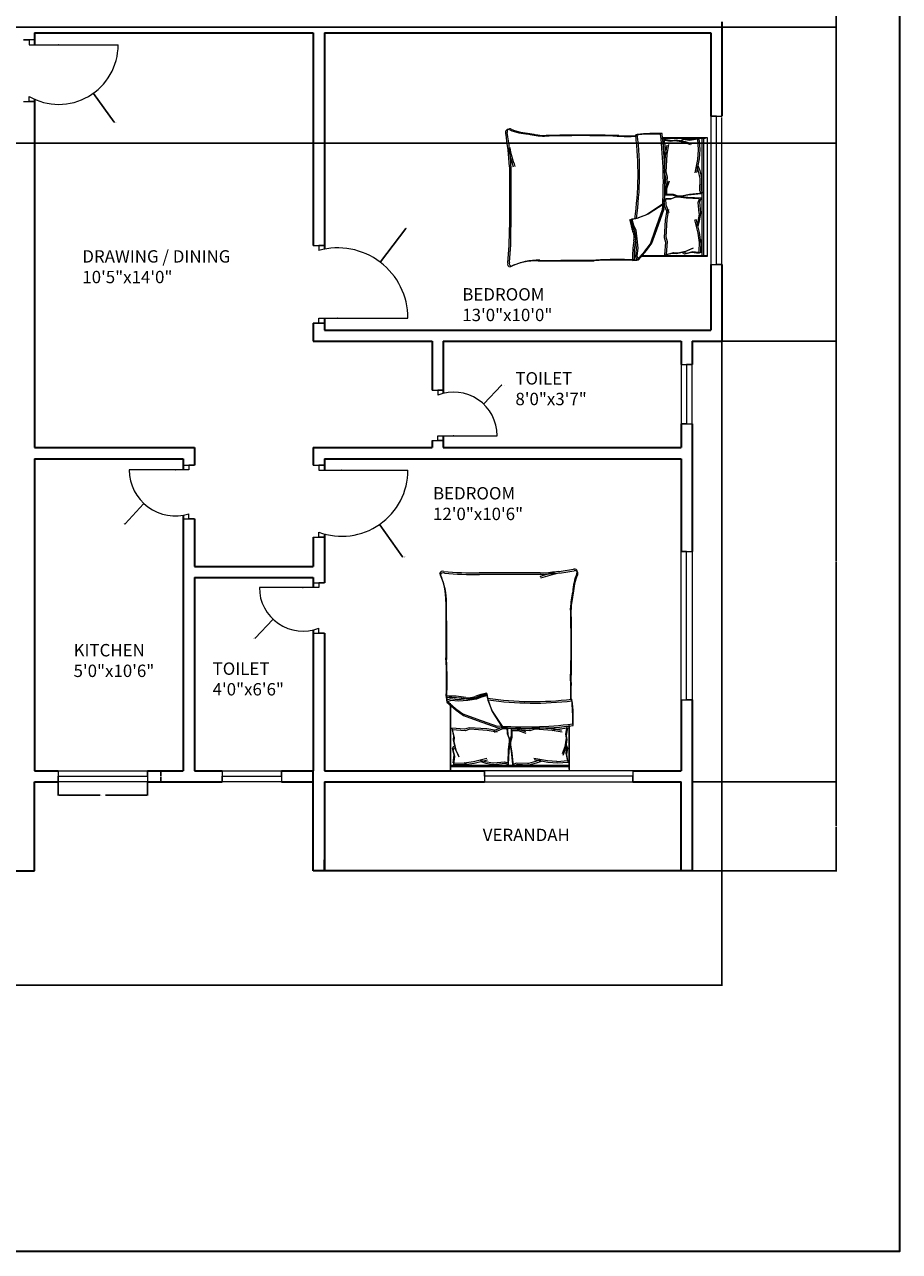
# Model space of a CAD drawing. Units: inches. Extents: x 1937 to 2996, y 1402 to 2323.
# Tile 9 of 10: x 2643 to 2996, y 1402 to 1897. Entities that reach past the tile are written whole.
import ezdxf

# ---------------------------------------------------------------- set-up
doc = ezdxf.new("R2010")
doc.units = ezdxf.units.IN
for name, color, linetype, lineweight in [('A-ANNO-DIMS', 2, 'Continuous', 18), ('A-ANNO-TTLB', 7, 'Continuous', 35), ('A-AREA-IDEN', 7, 'Continuous', 18), ('A-DOOR', 11, 'Continuous', 18), ('A-FURN', 8, 'Continuous', 13), ('A-GLAZ', 141, 'Continuous', 18), ('A-WALL', 7, 'Continuous', 35)]:
    doc.layers.add(name, color=color, linetype=linetype, lineweight=lineweight)
doc.styles.get("Standard").update_dxf_attribs({"font": 'arial.ttf'})
doc.dimstyles.get("Standard").update_dxf_attribs({"dimtxt": 0.18, "dimasz": 0.18, "dimexe": 0.18, "dimexo": 0.0625, "dimgap": 0.09, "dimtad": 0, "dimtih": 1, "dimtoh": 1, "dimdec": 4, "dimzin": 0, "dimdsep": 46, "dimtxsty": 'Standard', "dimcen": 0.09, "dimadec": 0, "dimazin": 0, "dimtfac": 1, "dimtdec": 4, "dimtofl": 0, "dimtmove": 0, "dimatfit": 3, "dimfxl": 1, "dimtolj": 1, "dimtzin": 0, "dimarcsym": 0})

# ---------------------------------------------------------------- blocks, each defined once
blk = doc.blocks.new('BED-DOUBLE')
for p, q in [((-24.01, -18.11), (-24.01, 0)), ((-24.01, -18.11), (-24.01, 0)), ((-24.01, 0), (24.01, 0)), ((23.78, 0), (23.78, -26.61)), ((23.78, 0), (23.78, -26.61)), ((24.01, 0), (24.01, -0.64)), ((-24.01, -1.53), (23.78, -1.53)), ((-24.01, -1.53), (23.78, -1.53)), ((-23.78, -18.75), (-23.78, -0.64)), ((-23.78, -18.75), (-23.78, -0.64)), ((-23.78, -2.17), (24.01, -2.17)), ((-23.78, -2.17), (24.01, -2.17)), ((-23.59, -3.34), (-19.3, -3.01)), ((-23.59, -3.34), (-19.31, -3.01)), ((-23.59, -3.32), (-23.01, -6.5)), ((-23.59, -3.32), (-23.01, -6.5)), ((-23.36, -3.98), (-19.08, -3.65)), ((-23.36, -3.98), (-19.08, -3.65)), ((-23.36, -3.96), (-22.78, -7.14)), ((-23.36, -3.96), (-22.78, -7.14)), ((-19.31, -3.01), (-19.2, -3.03)), ((-19.3, -3.01), (-19.2, -3.03)), ((-19.2, -3.03), (-15.38, -3.32)), ((-19.2, -3.03), (-15.38, -3.32)), ((-19.08, -3.65), (-18.97, -3.67)), ((-19.08, -3.65), (-18.97, -3.67)), ((-18.97, -3.67), (-15.15, -3.96)), ((-18.97, -3.67), (-15.15, -3.96)), ((-15.38, -3.32), (-9.88, -4.33)), ((-15.38, -3.32), (-9.88, -4.33)), ((-15.15, -3.96), (-9.65, -4.97)), ((-15.15, -3.96), (-9.65, -4.97)), ((-12.63, -3.75), (-10.61, -3.03)), ((-12.63, -3.75), (-10.61, -3.03)), ((-12.4, -4.39), (-10.38, -3.67)), ((-12.4, -4.39), (-10.38, -3.67)), ((-10.61, -3.03), (-7.71, -2.3)), ((-10.61, -3.03), (-7.71, -2.3)), ((-10.38, -3.67), (-7.49, -2.94)), ((-10.38, -3.67), (-7.49, -2.94)), ((-7.71, -2.3), (-7.39, -2.3)), ((-7.71, -2.3), (-7.39, -2.3)), ((-7.49, -2.94), (-7.16, -2.94)), ((-7.49, -2.94), (-7.16, -2.94)), ((-7.39, -2.3), (-2.95, -2.45)), ((-7.39, -2.3), (-2.95, -2.45)), ((-7.16, -2.94), (-2.72, -3.09)), ((-7.16, -2.94), (-2.72, -3.09)), ((-2.95, -2.45), (-1.5, -1.87)), ((-2.95, -2.45), (-1.5, -1.87)), ((-2.72, -3.09), (-1.27, -2.51)), ((-2.72, -3.09), (-1.27, -2.51)), ((-1.5, -1.87), (-0.92, -7.22)), ((-1.5, -1.87), (-0.92, -7.22)), ((-1.27, -2.51), (-0.7, -7.86)), ((-1.27, -2.51), (-0.7, -7.86)), ((0.49, -2.49), (0.25, -7.87)), ((0.49, -2.49), (0.25, -7.87)), ((0.72, -3.13), (0.48, -8.51)), ((0.72, -3.13), (0.48, -8.51)), ((1.97, -2.98), (0.49, -2.49)), ((1.97, -2.98), (0.49, -2.49)), ((2.2, -3.62), (0.72, -3.13)), ((2.2, -3.62), (0.72, -3.13)), ((6.4, -2.56), (1.97, -2.98)), ((6.4, -2.56), (1.97, -2.98)), ((6.63, -3.2), (2.2, -3.62)), ((6.63, -3.2), (2.2, -3.62)), ((6.72, -2.54), (6.4, -2.56)), ((6.72, -2.54), (6.4, -2.56)), ((6.95, -3.18), (6.63, -3.2)), ((6.95, -3.18), (6.63, -3.2)), ((9.65, -3.08), (6.72, -2.54)), ((9.65, -3.08), (6.72, -2.54)), ((9.88, -3.72), (6.95, -3.18)), ((9.88, -3.72), (6.95, -3.18)), ((14.43, -3.07), (9.01, -4.42)), ((14.43, -3.07), (9.01, -4.42)), ((14.66, -3.71), (9.24, -5.06)), ((14.66, -3.71), (9.24, -5.06)), ((11.72, -3.67), (9.65, -3.08)), ((11.72, -3.67), (9.65, -3.08)), ((11.94, -4.31), (9.88, -3.72)), ((11.94, -4.31), (9.88, -3.72)), ((18.23, -2.54), (14.43, -3.07)), ((18.23, -2.54), (14.43, -3.07)), ((18.46, -3.18), (14.66, -3.71)), ((18.46, -3.18), (14.66, -3.71)), ((22.63, -2.56), (17.23, -2.46)), ((17.23, -2.46), (18.23, -2.54)), ((22.63, -2.56), (17.23, -2.46)), ((17.23, -2.46), (18.23, -2.54)), ((22.86, -3.2), (17.45, -3.1)), ((17.45, -3.1), (18.46, -3.18)), ((22.86, -3.2), (17.45, -3.1)), ((17.45, -3.1), (18.46, -3.18)), ((22.63, -2.56), (22.25, -5.77)), ((22.63, -2.56), (22.25, -5.77)), ((22.86, -3.2), (22.48, -6.41)), ((22.86, -3.2), (22.48, -6.41)), ((24.01, -0.64), (24.01, -27.25)), ((24.01, -0.64), (24.01, -27.25)), ((-23.01, -6.5), (-23.45, -9.1)), ((-23.01, -6.5), (-23.45, -9.1)), ((-23.45, -9.1), (-22.87, -10.11)), ((-23.45, -9.1), (-22.87, -10.11)), ((-22.78, -7.14), (-23.22, -9.74)), ((-22.78, -7.14), (-23.22, -9.74)), ((-23.22, -9.74), (-22.64, -10.75)), ((-23.22, -9.74), (-22.64, -10.75)), ((-23.01, -12.57), (-22.43, -8.96)), ((-23.01, -12.57), (-22.43, -8.96)), ((-22.78, -13.21), (-22.2, -9.59)), ((-22.78, -13.21), (-22.21, -9.59)), ((-22.43, -8.96), (-21.42, -6.21)), ((-22.43, -8.96), (-21.42, -6.21)), ((-22.21, -9.59), (-21.19, -6.85)), ((-22.2, -9.59), (-21.19, -6.85)), ((-0.92, -7.22), (-0.35, -10.4)), ((-0.92, -7.22), (-0.35, -10.4)), ((-0.7, -7.86), (-0.12, -11.04)), ((-0.7, -7.86), (-0.12, -11.04)), ((0.25, -7.87), (-0.13, -11.08)), ((0.25, -7.87), (-0.13, -11.08)), ((0.48, -8.51), (0.1, -11.72)), ((0.48, -8.51), (0.1, -11.72)), ((21.83, -8.26), (20.64, -5.58)), ((21.82, -8.26), (20.64, -5.58)), ((22.05, -8.9), (20.87, -6.22)), ((22.05, -8.9), (20.87, -6.22)), ((22.63, -11.83), (21.82, -8.26)), ((22.63, -11.83), (21.83, -8.26)), ((22.86, -12.47), (22.05, -8.9)), ((22.86, -12.47), (22.05, -8.9)), ((22.25, -5.77), (22.84, -8.34)), ((22.25, -5.77), (22.84, -8.34)), ((22.84, -8.34), (22.33, -9.38)), ((22.84, -8.34), (22.33, -9.38)), ((22.48, -6.41), (23.07, -8.98)), ((22.48, -6.41), (23.07, -8.98)), ((23.07, -8.98), (22.56, -10.02)), ((23.07, -8.98), (22.56, -10.02)), ((-23.3, -17.34), (-22.72, -14.16)), ((-23.3, -17.34), (-22.72, -14.16)), ((-23.07, -17.98), (-22.49, -14.8)), ((-23.07, -17.98), (-22.49, -14.8)), ((-22.72, -14.16), (-23.01, -12.57)), ((-22.72, -14.16), (-23.01, -12.57)), ((-22.49, -14.8), (-22.78, -13.21)), ((-22.49, -14.8), (-22.78, -13.21)), ((-0.35, -11.7), (-0.92, -13.58)), ((-0.35, -11.7), (-0.92, -13.58)), ((-0.92, -13.58), (-0.92, -16.26)), ((-0.92, -13.58), (-0.92, -16.26)), ((-0.12, -12.34), (-0.7, -14.22)), ((-0.12, -12.34), (-0.7, -14.22)), ((-0.7, -14.22), (-0.7, -16.9)), ((-0.7, -14.22), (-0.7, -16.9)), ((-0.35, -10.4), (-0.35, -11.7)), ((-0.35, -10.4), (-0.35, -11.7)), ((-0.13, -11.08), (-0.05, -12.38)), ((-0.13, -11.08), (-0.05, -12.38)), ((-0.12, -11.04), (-0.12, -12.34)), ((-0.12, -11.04), (-0.12, -12.34)), ((-0.05, -12.38), (0.65, -14.22)), ((-0.05, -12.38), (0.65, -14.22)), ((0.1, -11.72), (0.18, -13.02)), ((0.1, -11.72), (0.18, -13.02)), ((0.18, -13.02), (0.87, -14.86)), ((0.18, -13.02), (0.87, -14.86)), ((0.65, -14.22), (0.81, -16.89)), ((0.65, -14.22), (0.81, -16.89)), ((0.87, -14.86), (1.04, -17.53)), ((0.87, -14.86), (1.04, -17.53)), ((22.44, -13.43), (22.63, -11.83)), ((22.44, -13.43), (22.63, -11.83)), ((23.21, -16.57), (22.44, -13.43)), ((23.21, -16.57), (22.44, -13.43)), ((22.67, -14.07), (22.86, -12.47)), ((22.67, -14.07), (22.86, -12.47)), ((23.44, -17.21), (22.67, -14.07)), ((23.44, -17.21), (22.67, -14.07)), ((-18.2, -16.62), (-23.3, -17.34)), ((-18.2, -16.62), (-23.3, -17.34)), ((-17.98, -17.26), (-23.07, -17.98)), ((-17.98, -17.26), (-23.07, -17.98)), ((-21.1, -15.63), (-17.07, -16.3)), ((-21.1, -15.63), (-17.07, -16.3)), ((-20.87, -16.27), (-16.84, -16.93)), ((-20.87, -16.27), (-16.84, -16.93)), ((-17.07, -16.3), (-18.2, -16.62)), ((-17.07, -16.3), (-18.2, -16.62)), ((-16.84, -16.93), (-17.98, -17.26)), ((-16.84, -16.93), (-17.98, -17.26)), ((-17.07, -16.3), (-10.06, -16.73)), ((-17.07, -16.3), (-10.06, -16.73)), ((-16.84, -16.93), (-9.83, -17.37)), ((-16.84, -16.93), (-9.83, -17.37)), ((-10.06, -16.73), (-8.1, -16.17)), ((-10.06, -16.73), (-8.1, -16.17)), ((-9.83, -17.37), (-7.87, -16.81)), ((-9.83, -17.37), (-7.87, -16.81)), ((-8.1, -16.17), (-2.97, -16.57)), ((-8.1, -16.17), (-2.97, -16.57)), ((-7.87, -16.81), (-2.74, -17.21)), ((-7.87, -16.81), (-2.74, -17.21)), ((-3.38, -16.26), (-6.53, -15.17)), ((-3.38, -16.26), (-6.53, -15.17)), ((-3.15, -16.9), (-6.3, -15.81)), ((-3.15, -16.9), (-6.3, -15.81)), ((-0.92, -16.26), (-3.38, -16.26)), ((-0.92, -16.26), (-3.38, -16.26)), ((-0.7, -16.9), (-3.15, -16.9)), ((-0.7, -16.9), (-3.15, -16.9)), ((0.81, -16.89), (3.27, -16.74)), ((0.81, -16.89), (3.27, -16.74)), ((1.04, -17.53), (3.49, -17.38)), ((1.04, -17.53), (3.49, -17.38)), ((2.77, -17.38), (6.97, -23.88)), ((2.77, -17.38), (6.96, -23.88)), ((3, -18.02), (7.19, -24.52)), ((3, -18.02), (7.19, -24.52)), ((3.27, -16.74), (6.34, -15.45)), ((3.27, -16.74), (6.34, -15.45)), ((3.49, -17.38), (6.56, -16.09)), ((3.49, -17.38), (6.56, -16.09)), ((13.16, -20.32), (4.82, -17.38)), ((13.16, -20.32), (4.82, -17.38)), ((13.39, -20.96), (5.05, -18.02)), ((13.39, -20.96), (5.05, -18.02)), ((5.08, -15.63), (9.11, -16.3)), ((5.08, -15.63), (9.11, -16.3)), ((5.31, -16.27), (9.34, -16.93)), ((5.31, -16.27), (9.34, -16.93)), ((9.11, -16.3), (16.12, -16.73)), ((9.11, -16.3), (16.12, -16.73)), ((9.34, -16.93), (16.35, -17.37)), ((9.34, -16.93), (16.35, -17.37)), ((16.12, -16.73), (18.08, -16.17)), ((16.12, -16.73), (18.08, -16.17)), ((16.35, -17.37), (18.31, -16.81)), ((16.35, -17.37), (18.31, -16.81)), ((18.08, -16.17), (23.21, -16.57)), ((18.08, -16.17), (23.21, -16.57)), ((18.31, -16.81), (23.44, -17.21)), ((18.31, -16.81), (23.44, -17.21)), ((6.96, -23.88), (8.67, -28.37)), ((6.97, -23.88), (8.67, -28.37)), ((7.19, -24.52), (8.9, -29)), ((7.19, -24.52), (8.9, -29)), ((18.74, -22.33), (13.16, -20.32)), ((18.74, -22.33), (13.16, -20.32)), ((18.96, -22.97), (13.39, -20.96)), ((18.96, -22.97), (13.39, -20.96)), ((21.68, -24.5), (18.74, -22.33)), ((21.68, -24.5), (18.74, -22.33)), ((21.91, -25.13), (18.96, -22.97)), ((21.91, -25.13), (18.96, -22.97)), ((25.38, -27.75), (21.68, -24.5)), ((25.38, -27.75), (21.68, -24.5)), ((8.67, -28.37), (8.98, -30.38)), ((8.67, -28.37), (8.98, -30.38)), ((8.9, -29), (9.21, -31.02)), ((8.9, -29), (9.21, -31.02)), ((11.46, -29.76), (13.47, -28.83)), ((11.46, -29.76), (13.47, -28.83)), ((11.68, -30.4), (13.7, -29.47)), ((11.68, -30.4), (13.7, -29.47)), ((13.47, -28.83), (16.88, -28.37)), ((13.47, -28.83), (16.88, -28.37)), ((13.7, -29.47), (17.11, -29)), ((13.7, -29.47), (17.1, -29)), ((16.88, -28.37), (20.75, -28.06)), ((16.88, -28.37), (20.75, -28.06)), ((17.1, -29), (20.98, -28.69)), ((17.11, -29), (20.98, -28.69)), ((20.75, -28.06), (23.85, -28.37)), ((20.75, -28.06), (23.85, -28.37)), ((20.98, -28.69), (24.07, -29)), ((20.98, -28.69), (24.07, -29)), ((25.61, -28.39), (21.91, -25.13)), ((25.61, -28.39), (21.91, -25.13)), ((23.85, -28.37), (25.38, -27.75)), ((23.85, -28.37), (25.38, -27.75)), ((24.07, -29), (25.61, -28.39)), ((24.07, -29), (25.61, -28.39)), ((25.46, -29.49), (25.38, -27.75, 3.87)), ((25.46, -29.49), (25.38, -27.75, 3.87)), ((25.69, -30.13), (25.61, -28.39, 3.87)), ((25.69, -30.13), (25.61, -28.39, 3.87)), ((8.98, -30.38), (11.46, -29.76)), ((8.98, -30.38), (11.46, -29.76)), ((9.21, -31.02), (11.68, -30.4)), ((9.21, -31.02), (11.68, -30.4)), ((-12.42, -79.25), (12.19, -79.25)), ((-12.42, -79.25), (12.19, -79.25)), ((-12.19, -79.88), (12.42, -79.88)), ((-12.19, -79.88), (12.42, -79.88))]:
    blk.add_line(p, q)
for centre, radius, start, end in [((57.68, -20.1), 83.31, 178.7218, 185.604), ((57.68, -20.1), 83.31, 178.7218, 185.604), ((-6.13, -182.05), 164.97, 86.0865, 96.7821), ((-6.13, -182.05), 164.97, 86.0865, 96.7821), ((57.91, -20.74), 83.31, 178.7218, 185.604), ((57.91, -20.74), 83.31, 178.7218, 185.604), ((-5.9, -182.69), 164.97, 86.0865, 96.7821), ((-5.9, -182.69), 164.97, 86.0865, 96.7821), ((-9.73, -156.32), 129.02, 81.7845, 96.9006), ((-9.73, -156.32), 129.02, 81.7845, 96.9006), ((-9.5, -156.96), 129.02, 81.7845, 96.9006), ((-9.5, -156.96), 129.02, 81.7845, 96.9006), ((-194.79, -31.17), 170.11, 358.4762, 1.0082), ((-194.79, -31.17), 170.11, 358.4762, 1.0082), ((-194.56, -31.81), 170.11, 358.4762, 1.0082), ((-194.56, -31.81), 170.11, 358.4762, 1.0082), ((3.67, -1.48), 29.65, 280.6617, 289.8806), ((3.67, -1.48), 29.65, 280.6617, 289.8806), ((16.26, -35.07), 6.22, 78.6608, 113.7384), ((16.26, -35.07), 6.22, 78.6608, 113.7384), ((16.49, -35.71), 6.22, 78.6608, 113.7384), ((16.49, -35.71), 6.22, 78.6608, 113.7384), ((23.84, 6.66), 36.18, 259.8763, 272.5657), ((23.84, 6.66), 36.18, 259.8763, 272.5657), ((24.07, 6.02), 36.18, 259.8763, 272.5657), ((24.07, 6.02), 36.18, 259.8763, 272.5657), ((154.78, -36.32), 129.5, 176.9791, 183.8365), ((154.78, -36.32), 129.5, 176.9791, 183.8365), ((9.15, -30.44), 0.185, 160.2464, 271.1377), ((9.15, -30.44), 0.185, 160.2464, 271.1377), ((9.38, -31.08), 0.185, 160.2464, 271.1377), ((9.38, -31.08), 0.185, 160.2464, 271.1377), ((3.9, -2.12), 29.65, 280.6617, 289.8806), ((3.9, -2.12), 29.65, 280.6617, 289.8806), ((155.01, -36.95), 129.5, 176.9791, 183.8365), ((155.01, -36.95), 129.5, 176.9791, 183.8365), ((457.34, -50.61), 482.31, 178.2277, 181.7185), ((457.34, -50.61), 482.31, 178.2277, 181.7185), ((457.57, -51.25), 482.31, 178.2277, 181.7185), ((457.57, -51.25), 482.31, 178.2277, 181.7185), ((-4536.23, -67.82), 4561.86, 0.00217, 0.28689), ((-4536.23, -67.82), 4561.86, 0.00217, 0.28689), ((-4536, -68.46), 4561.86, 0.00217, 0.28689), ((-4536, -68.46), 4561.86, 0.00217, 0.28689), ((-54.38, -64.52), 29.63, 346.0648, 358.9113), ((-54.38, -64.52), 29.63, 346.0648, 358.9113), ((-54.16, -65.15), 29.63, 346.0648, 358.9113), ((-54.16, -65.15), 29.63, 346.0648, 358.9113), ((48.67, -68.67), 23.07, 177.4714, 206.4681), ((48.67, -68.67), 23.07, 177.4714, 206.4681), ((48.9, -69.31), 23.07, 177.4714, 206.4681), ((48.9, -69.31), 23.07, 177.4714, 206.4681), ((-49.14, -70.28), 23.56, 337.9751, 356.652), ((-49.14, -70.28), 23.56, 337.9751, 356.652), ((-48.92, -70.91), 23.56, 337.9751, 356.652), ((-48.92, -70.91), 23.56, 337.9751, 356.652), ((-26.4, -79.72), 1.09, 146.1736, 293.4781), ((-26.4, -79.72), 1.09, 146.1736, 293.4781), ((-6.06, -200.84), 121.76, 92.9958, 99.4091), ((-6.06, -200.84), 121.76, 92.9958, 99.4091), ((-44.71, 23.71), 106.46, 283.3832, 287.7053), ((-44.71, 23.71), 106.46, 283.3832, 287.7053), ((-44.48, 23.07), 106.46, 283.3832, 287.7053), ((-44.48, 23.07), 106.46, 283.3832, 287.7053), ((13.67, -212.28), 133.04, 84.4998, 90.6351), ((13.67, -212.28), 133.04, 84.4998, 90.6351), ((26.93, -78.87), 1.1, 242.6588, 356.02), ((26.93, -78.87), 1.1, 242.6588, 356.02), ((-26.17, -80.36), 1.09, 146.1736, 293.4781), ((-26.17, -80.36), 1.09, 146.1736, 293.4781), ((-5.83, -201.48), 121.76, 92.9958, 99.4091), ((-5.83, -201.48), 121.76, 92.9958, 99.4091), ((13.9, -212.92), 133.04, 84.4998, 90.6351), ((13.9, -212.92), 133.04, 84.4998, 90.6351), ((27.15, -79.51), 1.1, 242.6588, 356.02), ((27.15, -79.51), 1.1, 242.6588, 356.02)]:
    blk.add_arc(centre, radius, start, end)
blk = doc.blocks.new('WINDOW-60IN')
for p, q in [((0, 2.25), (0, -2.25)), ((0, 2.25), (60, 2.25)), ((0, -2.25), (0, 0)), ((0, 0), (60, 0)), ((60, 0), (60, 2.25)), ((60, 2.25), (60, -2.25)), ((60, -2.25), (0, -2.25))]:
    blk.add_line(p, q)
blk = doc.blocks.new('WINDOW-24IN')
for p, q in [((0, -2.25), (0, 2.25)), ((0, 2.25), (0, 0)), ((24, 2.25), (0, 2.25)), ((0, 0), (24, 0)), ((24, -2.25), (24, 2.25)), ((24, 0), (24, -2.25)), ((0, -2.25), (24, -2.25))]:
    blk.add_line(p, q)
blk = doc.blocks.new('WINDOW-36IN')
for p, q in [((0, 2.25), (0, -2.25)), ((0, 2.25), (36, 2.25)), ((36, 0), (36, 2.25)), ((36, 2.25), (36, -2.25)), ((0, -2.25), (0, 0)), ((0, 0), (36, 0)), ((36, -2.25), (0, -2.25))]:
    blk.add_line(p, q)
blk = doc.blocks.new('*D15')
at = {"layer": 'A-ANNO-DIMS', "color": 0, "lineweight": -2, "transparency": 16777216}
for p, q in [((2656.2, 1591.24), (2656.2, 1585.73)), ((2692.2, 1591.24), (2692.2, 1585.73)), ((2656.38, 1585.91), (2673.09, 1585.91)), ((2692.02, 1585.91), (2675.32, 1585.91))]:
    blk.add_line(p, q, dxfattribs=at)
at = {"layer": 'A-ANNO-DIMS', "color": 0, "transparency": 16777216}
for points in [[(2656.38, 1585.94), (2656.38, 1585.88), (2656.2, 1585.91)], [(2692.02, 1585.94), (2692.02, 1585.88), (2692.2, 1585.91)]]:
    blk.add_solid(points, dxfattribs=at)
at = {"layer": 'Defpoints', "color": 0, "transparency": 16777216}
for p in [(2656.2, 1591.31), (2692.2, 1591.31), (2692.2, 1585.91)]:
    blk.add_point(p, dxfattribs=at)
at = {"layer": 'A-ANNO-DIMS', "color": 0, "transparency": 16777216, "insert": (2674.2, 1585.91), "char_height": 0.18, "attachment_point": 5}
blk.add_mtext('\\A1;WINDOW 36 TYP.', dxfattribs=at)
blk = doc.blocks.new('*D16')
at = {"layer": 'A-ANNO-DIMS', "color": 0, "lineweight": -2, "transparency": 16777216}
for p, q in [((2692.27, 1595.81), (2697.78, 1595.81)), ((2692.27, 1591.31), (2697.78, 1591.31)), ((2697.6, 1595.63), (2697.6, 1593.74)), ((2697.6, 1591.49), (2697.6, 1593.37))]:
    blk.add_line(p, q, dxfattribs=at)
at = {"layer": 'A-ANNO-DIMS', "color": 0, "transparency": 16777216}
for points in [[(2697.57, 1595.63), (2697.63, 1595.63), (2697.6, 1595.81)], [(2697.57, 1591.49), (2697.63, 1591.49), (2697.6, 1591.31)]]:
    blk.add_solid(points, dxfattribs=at)
at = {"layer": 'Defpoints', "color": 0, "transparency": 16777216}
for p in [(2692.2, 1595.81), (2697.6, 1595.81), (2692.2, 1591.31)]:
    blk.add_point(p, dxfattribs=at)
at = {"layer": 'A-ANNO-DIMS', "color": 0, "transparency": 16777216, "insert": (2697.6, 1593.56), "char_height": 0.18, "attachment_point": 5}
blk.add_mtext('\\A1;5 TYP.', dxfattribs=at)
blk = doc.blocks.new('*D23')
at = {"layer": 'A-ANNO-DIMS', "color": 0, "lineweight": -2, "transparency": 16777216}
for p, q in [((2010.65, 1769.24), (2010.65, 1508.98)), ((2924.15, 1769.24), (2924.15, 1508.98)), ((2010.83, 1509.16), (2467, 1509.16)), ((2923.97, 1509.16), (2467.79, 1509.16))]:
    blk.add_line(p, q, dxfattribs=at)
at = {"layer": 'A-ANNO-DIMS', "color": 0, "transparency": 16777216}
for points in [[(2010.83, 1509.19), (2010.83, 1509.13), (2010.65, 1509.16)], [(2923.97, 1509.19), (2923.97, 1509.13), (2924.15, 1509.16)]]:
    blk.add_solid(points, dxfattribs=at)
at = {"layer": 'Defpoints', "color": 0, "transparency": 16777216}
for p in [(2010.65, 1769.31), (2924.15, 1769.31), (2924.15, 1509.16)]:
    blk.add_point(p, dxfattribs=at)
at = {"layer": 'A-ANNO-DIMS', "color": 0, "transparency": 16777216, "insert": (2467.4, 1509.16), "char_height": 0.18, "attachment_point": 5}
blk.add_mtext('\\A1;913.5', dxfattribs=at)
blk = doc.blocks.new('*D37')
at = {"layer": 'A-ANNO-DIMS', "color": 0, "lineweight": -2, "transparency": 16777216}
for p, q in [((2455.84, 1896.06), (2970.48, 1896.06)), ((2970.3, 1895.88), (2970.3, 1872.86)), ((2970.3, 1849.49), (2970.3, 1872.5)), ((2455.84, 1849.31), (2970.48, 1849.31))]:
    blk.add_line(p, q, dxfattribs=at)
at = {"layer": 'A-ANNO-DIMS', "color": 0, "transparency": 16777216}
for points in [[(2970.27, 1895.88), (2970.33, 1895.88), (2970.3, 1896.06)], [(2970.27, 1849.49), (2970.33, 1849.49), (2970.3, 1849.31)]]:
    blk.add_solid(points, dxfattribs=at)
at = {"layer": 'Defpoints', "color": 0, "transparency": 16777216}
for p in [(2455.77, 1896.06), (2455.77, 1849.31), (2970.3, 1849.31)]:
    blk.add_point(p, dxfattribs=at)
at = {"layer": 'A-ANNO-DIMS', "color": 0, "transparency": 16777216, "insert": (2970.3, 1872.68), "char_height": 0.18, "attachment_point": 5}
blk.add_mtext('\\A1;46.75', dxfattribs=at)
blk = doc.blocks.new('*D39')
at = {"layer": 'A-ANNO-DIMS', "color": 0, "lineweight": -2, "transparency": 16777216}
for p, q in [((2912.21, 1591.31), (2970.48, 1591.31)), ((2970.3, 1591.13), (2970.3, 1573.49)), ((2970.3, 1555.49), (2970.3, 1573.12)), ((2912.21, 1555.31), (2970.48, 1555.31))]:
    blk.add_line(p, q, dxfattribs=at)
at = {"layer": 'A-ANNO-DIMS', "color": 0, "transparency": 16777216}
for points in [[(2970.27, 1591.13), (2970.33, 1591.13), (2970.3, 1591.31)], [(2970.27, 1555.49), (2970.33, 1555.49), (2970.3, 1555.31)]]:
    blk.add_solid(points, dxfattribs=at)
at = {"layer": 'Defpoints', "color": 0, "transparency": 16777216}
for p in [(2912.15, 1591.31), (2970.3, 1591.31), (2912.15, 1555.31)]:
    blk.add_point(p, dxfattribs=at)
at = {"layer": 'A-ANNO-DIMS', "color": 0, "transparency": 16777216, "insert": (2970.3, 1573.31), "char_height": 0.18, "attachment_point": 5}
blk.add_mtext('\\A1;36', dxfattribs=at)
blk = doc.blocks.new('*D40')
at = {"layer": 'A-ANNO-DIMS', "color": 0, "lineweight": -2, "transparency": 16777216}
for p, q in [((2912.21, 1769.31), (2970.48, 1769.31)), ((2970.3, 1769.13), (2970.3, 1680.49)), ((2970.3, 1591.49), (2970.3, 1680.12)), ((2912.21, 1591.31), (2970.48, 1591.31))]:
    blk.add_line(p, q, dxfattribs=at)
at = {"layer": 'A-ANNO-DIMS', "color": 0, "transparency": 16777216}
for points in [[(2970.27, 1769.13), (2970.33, 1769.13), (2970.3, 1769.31)], [(2970.27, 1591.49), (2970.33, 1591.49), (2970.3, 1591.31)]]:
    blk.add_solid(points, dxfattribs=at)
at = {"layer": 'Defpoints', "color": 0, "transparency": 16777216}
for p in [(2912.15, 1769.31), (2970.3, 1769.31), (2912.15, 1591.31)]:
    blk.add_point(p, dxfattribs=at)
at = {"layer": 'A-ANNO-DIMS', "color": 0, "transparency": 16777216, "insert": (2970.3, 1680.31), "char_height": 0.18, "attachment_point": 5}
blk.add_mtext('\\A1;178', dxfattribs=at)
blk = doc.blocks.new('*D41')
at = {"layer": 'A-ANNO-DIMS', "color": 0, "lineweight": -2, "transparency": 16777216}
for p, q in [((2924.21, 2022.81), (2970.48, 2022.81)), ((2970.3, 2022.63), (2970.3, 1896.24)), ((2970.3, 1769.49), (2970.3, 1895.87)), ((2924.21, 1769.31), (2970.48, 1769.31))]:
    blk.add_line(p, q, dxfattribs=at)
at = {"layer": 'A-ANNO-DIMS', "color": 0, "transparency": 16777216}
for points in [[(2970.27, 2022.63), (2970.33, 2022.63), (2970.3, 2022.81)], [(2970.27, 1769.49), (2970.33, 1769.49), (2970.3, 1769.31)]]:
    blk.add_solid(points, dxfattribs=at)
at = {"layer": 'Defpoints', "color": 0, "transparency": 16777216}
for p in [(2924.15, 2022.81), (2970.3, 2022.81), (2924.15, 1769.31)]:
    blk.add_point(p, dxfattribs=at)
at = {"layer": 'A-ANNO-DIMS', "color": 0, "transparency": 16777216, "insert": (2970.3, 1896.06), "char_height": 0.18, "attachment_point": 5}
blk.add_mtext('\\A1;253.5', dxfattribs=at)
blk = doc.blocks.new('*D65')
at = {"layer": 'A-ANNO-DIMS', "color": 0, "lineweight": -2, "transparency": 16777216}
for p, q in [((2796.48, 1814.77), (2786.29, 1801.35)), ((2796.66, 1814.77), (2796.48, 1814.77)), ((2768.92, 1778.61), (2769.1, 1778.61)), ((2769.01, 1778.52), (2769.01, 1778.7))]:
    blk.add_line(p, q, dxfattribs=at)
at = {"layer": 'A-ANNO-DIMS', "color": 0, "transparency": 16777216}
blk.add_solid([(2786.27, 1801.37), (2786.31, 1801.33), (2786.18, 1801.21)], dxfattribs=at)
at = {"layer": 'Defpoints', "color": 0, "transparency": 16777216}
for p in [(2786.18, 1801.21), (2769.01, 1778.61)]:
    blk.add_point(p, dxfattribs=at)
at = {"layer": 'A-ANNO-DIMS', "color": 0, "transparency": 16777216, "insert": (2797.21, 1814.77), "char_height": 0.18, "attachment_point": 5}
blk.add_mtext('\\A1;R28.385', dxfattribs=at)
blk = doc.blocks.new('*D69')
at = {"layer": 'A-ANNO-DIMS', "color": 0, "lineweight": -2, "transparency": 16777216}
for p, q in [((2770.56, 1717.24), (2770.74, 1717.24)), ((2770.65, 1717.15), (2770.65, 1717.33)), ((2795.12, 1682.13), (2786.05, 1695.15)), ((2795.3, 1682.13), (2795.12, 1682.13))]:
    blk.add_line(p, q, dxfattribs=at)
at = {"layer": 'A-ANNO-DIMS', "color": 0, "transparency": 16777216}
blk.add_solid([(2786.07, 1695.17), (2786.02, 1695.13), (2785.95, 1695.3)], dxfattribs=at)
at = {"layer": 'Defpoints', "color": 0, "transparency": 16777216}
for p in [(2770.65, 1717.24), (2785.95, 1695.3)]:
    blk.add_point(p, dxfattribs=at)
at = {"layer": 'A-ANNO-DIMS', "color": 0, "transparency": 16777216, "insert": (2795.85, 1682.13), "char_height": 0.18, "attachment_point": 5}
blk.add_mtext('\\A1;R26.747', dxfattribs=at)
blk = doc.blocks.new('*D87')
at = {"layer": 'A-ANNO-DIMS', "color": 0, "lineweight": -2, "transparency": 16777216}
for p, q in [((2703.38, 1717.27), (2703.56, 1717.27)), ((2703.47, 1717.18), (2703.47, 1717.36)), ((2683.18, 1695.56), (2690.66, 1703.57)), ((2683, 1695.56), (2683.18, 1695.56))]:
    blk.add_line(p, q, dxfattribs=at)
at = {"layer": 'A-ANNO-DIMS', "color": 0, "transparency": 16777216}
blk.add_solid([(2690.64, 1703.59), (2690.69, 1703.55), (2690.79, 1703.7)], dxfattribs=at)
at = {"layer": 'Defpoints', "color": 0, "transparency": 16777216}
for p in [(2703.47, 1717.27), (2690.79, 1703.7)]:
    blk.add_point(p, dxfattribs=at)
at = {"layer": 'A-ANNO-DIMS', "color": 0, "transparency": 16777216, "insert": (2682.52, 1695.56), "char_height": 0.18, "attachment_point": 5}
blk.add_mtext('\\A1;R18.57', dxfattribs=at)
blk = doc.blocks.new('*D88')
at = {"layer": 'A-ANNO-DIMS', "color": 0, "lineweight": -2, "transparency": 16777216}
for p, q in [((2754.87, 1669.75), (2755.05, 1669.75)), ((2754.96, 1669.66), (2754.96, 1669.84)), ((2735.69, 1649.3), (2742.79, 1656.84)), ((2735.51, 1649.3), (2735.69, 1649.3))]:
    blk.add_line(p, q, dxfattribs=at)
at = {"layer": 'A-ANNO-DIMS', "color": 0, "transparency": 16777216}
blk.add_solid([(2742.77, 1656.86), (2742.81, 1656.82), (2742.92, 1656.97)], dxfattribs=at)
at = {"layer": 'Defpoints', "color": 0, "transparency": 16777216}
for p in [(2754.96, 1669.75), (2742.92, 1656.97)]:
    blk.add_point(p, dxfattribs=at)
at = {"layer": 'A-ANNO-DIMS', "color": 0, "transparency": 16777216, "insert": (2735.03, 1649.3), "char_height": 0.18, "attachment_point": 5}
blk.add_mtext('\\A1;R17.56', dxfattribs=at)
blk = doc.blocks.new('*D89')
at = {"layer": 'A-ANNO-DIMS', "color": 0, "lineweight": -2, "transparency": 16777216}
for p, q in [((2835.17, 1751.56), (2828.03, 1744.03)), ((2835.35, 1751.56), (2835.17, 1751.56)), ((2815.7, 1731.12), (2815.88, 1731.12)), ((2815.79, 1731.03), (2815.79, 1731.21))]:
    blk.add_line(p, q, dxfattribs=at)
at = {"layer": 'A-ANNO-DIMS', "color": 0, "transparency": 16777216}
blk.add_solid([(2828.01, 1744.05), (2828.05, 1744.01), (2827.9, 1743.9)], dxfattribs=at)
at = {"layer": 'Defpoints', "color": 0, "transparency": 16777216}
for p in [(2827.9, 1743.9), (2815.79, 1731.12)]:
    blk.add_point(p, dxfattribs=at)
at = {"layer": 'A-ANNO-DIMS', "color": 0, "transparency": 16777216, "insert": (2835.9, 1751.56), "char_height": 0.18, "attachment_point": 5}
blk.add_mtext('\\A1;R17.604', dxfattribs=at)
blk = doc.blocks.new('*D90')
at = {"layer": 'A-ANNO-DIMS', "color": 0, "lineweight": -2, "transparency": 16777216}
for p, q in [((2656.29, 1888.95), (2656.47, 1888.95)), ((2656.38, 1888.86), (2656.38, 1889.04)), ((2678.8, 1857.75), (2670.5, 1869.3)), ((2678.98, 1857.75), (2678.8, 1857.75))]:
    blk.add_line(p, q, dxfattribs=at)
at = {"layer": 'A-ANNO-DIMS', "color": 0, "transparency": 16777216}
blk.add_solid([(2670.52, 1869.32), (2670.48, 1869.29), (2670.4, 1869.45)], dxfattribs=at)
at = {"layer": 'Defpoints', "color": 0, "transparency": 16777216}
for p in [(2656.38, 1888.95), (2670.4, 1869.45)]:
    blk.add_point(p, dxfattribs=at)
at = {"layer": 'A-ANNO-DIMS', "color": 0, "transparency": 16777216, "insert": (2679.53, 1857.75), "char_height": 0.18, "attachment_point": 5}
blk.add_mtext('\\A1;R24.017', dxfattribs=at)

msp = doc.modelspace()

# ---------------------------------------------------------------- linework, layer by layer
at = {"layer": 'A-ANNO-TTLB'}
msp.add_lwpolyline([(1937.1125, 2323.2883), (2995.8132, 2323.2883), (2995.8132, 1401.6335), (1937.1125, 1401.6335)], close=True, dxfattribs=at)
at = {"layer": 'A-DOOR'}
for p, q in [((2646.6473, 1890.9534), (2642.1473, 1890.9534)), ((2642.1473, 1890.9534), (2644.3973, 1890.9534)), ((2644.3973, 1890.9534), (2644.3973, 1888.9534)), ((2644.3973, 1888.9534), (2680.3973, 1888.9534)), ((2642.1473, 1866.1389), (2646.6473, 1866.1389)), ((2644.3973, 1866.1389), (2644.3973, 1868.1389)), ((2646.6473, 1866.1389), (2644.3973, 1866.1389)), ((2759.1473, 1807.9501), (2763.6473, 1807.9501)), ((2763.6473, 1807.9501), (2761.3973, 1807.9501)), ((2761.3973, 1807.9501), (2761.3973, 1805.9501)), ((2763.6473, 1776.6052), (2759.1473, 1776.6052)), ((2759.1473, 1776.6052), (2763.6473, 1776.6052)), ((2761.3973, 1776.6052), (2761.3973, 1778.6052)), ((2761.3973, 1778.6052), (2797.3973, 1778.6052)), ((2763.6473, 1776.6052), (2761.3973, 1776.6052)), ((2807.1473, 1749.5251), (2811.6473, 1749.5251)), ((2811.6473, 1749.5251), (2809.3973, 1749.5251)), ((2809.3973, 1749.5251), (2809.3973, 1747.5251)), ((2809.3973, 1729.1246), (2809.3973, 1731.1246)), ((2809.3973, 1731.1246), (2833.3973, 1731.1246)), ((2807.1473, 1729.1246), (2811.6473, 1729.1246)), ((2811.6473, 1729.1246), (2809.3973, 1729.1246)), ((2708.8973, 1717.2682), (2684.8973, 1717.2682)), ((2706.6473, 1719.2682), (2711.1473, 1719.2682)), ((2711.1473, 1719.2682), (2708.8973, 1719.2682)), ((2708.8973, 1719.2682), (2708.8973, 1717.2682)), ((2759.1473, 1719.2395), (2763.6473, 1719.2395)), ((2763.6473, 1719.2395), (2761.3973, 1719.2395)), ((2761.3973, 1719.2395), (2761.3973, 1717.2395)), ((2761.3973, 1717.2395), (2797.3973, 1717.2395)), ((2763.6473, 1719.2395), (2763.6473, 1719.2395)), ((2706.6473, 1697.5088), (2711.1473, 1697.5088)), ((2708.8973, 1697.5088), (2708.8973, 1699.5088)), ((2711.1473, 1697.5088), (2708.8973, 1697.5088)), ((2759.1473, 1690.144), (2763.6473, 1690.144)), ((2761.3973, 1690.144), (2761.3973, 1692.144)), ((2763.6473, 1690.144), (2761.3973, 1690.144)), ((2759.1473, 1671.7534), (2763.6473, 1671.7534)), ((2763.6473, 1671.7534), (2761.3973, 1671.7534)), ((2761.3973, 1671.7534), (2761.3973, 1669.7534)), ((2761.3973, 1669.7534), (2737.3973, 1669.7534)), ((2759.1473, 1651.4159), (2763.6473, 1651.4159)), ((2761.3973, 1651.4159), (2761.3973, 1653.4159)), ((2763.6473, 1651.4159), (2761.3973, 1651.4159))]:
    msp.add_line(p, q, dxfattribs=at)
for centre, radius, start, end in [((2656.3801, 1888.9534), 24.0172, 240.071243, 360), ((2769.012, 1778.6052), 28.3853, 360, 105.560858), ((2815.7937, 1731.1246), 17.6036, 360, 111.30632), ((2703.4681, 1717.2682), 18.5707, 180, 286.998995), ((2770.6503, 1717.2395), 26.747, 249.760623, 0), ((2754.958, 1669.7534), 17.5607, 180, 291.511515)]:
    msp.add_arc(centre, radius, start, end, dxfattribs=at)
at = {"layer": 'A-GLAZ'}
for p, q in [((2921.8973, 1860.2229), (2919.6473, 1860.2229)), ((2919.6473, 1860.2229), (2924.1473, 1860.2229)), ((2919.6473, 1860.2229), (2919.6473, 1800.2229)), ((2921.8973, 1800.2229), (2921.8973, 1860.2229)), ((2924.1473, 1800.2229), (2924.1473, 1859.6039)), ((2919.6473, 1800.2229), (2924.1473, 1800.2229)), ((2924.1473, 1800.2229), (2921.8973, 1800.2229))]:
    msp.add_line(p, q, dxfattribs=at)
at = {"layer": 'A-WALL'}
for p, q in [((2924.1473, 1898.3061), (2924.1473, 1860.2229)), ((2646.6473, 1893.8061), (2759.1473, 1893.8061)), ((2646.6473, 1893.8061), (2646.6473, 1888.9534)), ((2759.1473, 1893.8061), (2759.1473, 1807.9501)), ((2763.6473, 1893.8061), (2763.6473, 1806.479)), ((2763.6473, 1893.8061), (2919.6473, 1893.8061)), ((2919.6473, 1893.8061), (2919.6473, 1860.2229)), ((2646.6473, 1866.9966), (2646.6473, 1726.3061)), ((2919.6473, 1800.2229), (2919.6473, 1773.8061)), ((2924.1473, 1800.2229), (2924.1473, 1769.3061)), ((2759.1473, 1776.6052), (2759.1473, 1769.3061)), ((2763.6473, 1778.6052), (2763.6473, 1773.8061)), ((2759.1473, 1769.3061), (2807.1473, 1769.3061)), ((2763.6473, 1773.8061), (2919.6473, 1773.8061)), ((2807.1473, 1769.3061), (2807.1473, 1749.5251)), ((2811.6473, 1769.3061), (2811.6473, 1748.233)), ((2811.6473, 1769.3061), (2907.6473, 1769.3061)), ((2907.6473, 1769.3061), (2907.6473, 1759.8951)), ((2912.1473, 1769.3061), (2912.1473, 1759.8951)), ((2912.1473, 1769.3061), (2924.1473, 1769.3061)), ((2907.6473, 1735.8951), (2907.6473, 1726.3061)), ((2912.1473, 1735.8951), (2912.1473, 1684.3814)), ((2811.6473, 1731.1246), (2811.6473, 1726.3061)), ((2646.6473, 1726.3061), (2711.1473, 1726.3061)), ((2711.1473, 1726.3061), (2711.1473, 1719.2682)), ((2759.1473, 1726.3061), (2759.1473, 1719.2395)), ((2759.1473, 1726.3061), (2807.1473, 1726.3061)), ((2807.1473, 1729.1246), (2807.1473, 1726.3061)), ((2811.6473, 1726.3061), (2907.6473, 1726.3061)), ((2646.6473, 1721.8061), (2706.6473, 1721.8061)), ((2646.6473, 1721.8061), (2646.6473, 1595.8061)), ((2706.6473, 1721.8061), (2706.6473, 1717.2682)), ((2763.6473, 1721.8061), (2763.6473, 1717.2395)), ((2763.6473, 1721.8061), (2907.6473, 1721.8061)), ((2907.6473, 1721.8061), (2907.6473, 1684.3814)), ((2706.6473, 1698.9716), (2706.6473, 1595.8061)), ((2711.1473, 1697.5088), (2711.1473, 1678.3061)), ((2759.1473, 1690.144), (2759.1473, 1678.3061)), ((2763.6473, 1691.4255), (2763.6473, 1671.7534)), ((2711.1473, 1678.3061), (2759.1473, 1678.3061)), ((2711.1473, 1673.8061), (2759.1473, 1673.8061)), ((2711.1473, 1673.8061), (2711.1473, 1595.8061)), ((2759.1473, 1673.8061), (2759.1473, 1669.7534)), ((2759.1473, 1652.6998), (2759.1473, 1595.8061)), ((2763.6473, 1651.4159), (2763.6473, 1595.8061)), ((2907.6473, 1624.3814), (2907.6473, 1595.8061)), ((2912.1473, 1624.3814), (2912.1473, 1591.3061)), ((2646.6473, 1595.8061), (2656.2044, 1595.8061)), ((2692.2044, 1595.8061), (2706.6473, 1595.8061)), ((2711.1473, 1595.8061), (2722.3271, 1595.8061)), ((2746.3271, 1595.8061), (2759.1473, 1595.8061)), ((2759.1473, 1555.3061), (2759.1473, 1595.8061)), ((2763.6473, 1595.8061), (2828.2339, 1595.8061)), ((2888.2339, 1595.8061), (2907.6473, 1595.8061)), ((2646.6473, 1591.3061), (2656.2044, 1591.3061)), ((2646.6473, 1555.3061), (2646.6473, 1591.3061)), ((2692.2044, 1591.3061), (2722.3271, 1591.3061)), ((2746.3271, 1591.3061), (2759.1473, 1591.3061)), ((2763.6473, 1591.3061), (2763.6473, 1555.3061)), ((2763.6473, 1591.3061), (2828.2339, 1591.3061)), ((2888.2339, 1591.3061), (2907.6473, 1591.3061)), ((2907.6473, 1555.3061), (2907.6473, 1591.3061)), ((2912.1473, 1591.3061), (2912.1473, 1555.3061)), ((2763.6473, 1555.3061), (2763.6473, 1559.8061)), ((2602.6116, 1555.3061), (2646.6473, 1555.3061)), ((2912.1473, 1555.3061), (2759.1473, 1555.3061))]:
    msp.add_line(p, q, dxfattribs=at)

# ---------------------------------------------------------------- block references
at = {"layer": 'A-FURN'}
for p, rotation in [((2918.2152, 1827.5684), 269.9999998331858), ((2838.5075, 1595.8061), 180)]:
    msp.add_blockref('BED-DOUBLE', p, dxfattribs=dict(at, rotation=rotation))
at = {"layer": 'A-GLAZ'}
for name, p, rotation in [('WINDOW-24IN', (2909.8973, 1759.8951), 270), ('WINDOW-60IN', (2909.8973, 1624.3814), 90)]:
    msp.add_blockref(name, p, dxfattribs=dict(at, rotation=rotation))
msp.add_blockref('WINDOW-36IN', (2656.2044, 1593.5561), dxfattribs=at)
at = {"layer": 'A-GLAZ', "extrusion": (0, 0, -1), "zscale": -1, "rotation": 180}
msp.add_blockref('WINDOW-24IN', (-2722.3271, 1593.5561), dxfattribs=at)
at = {"layer": 'A-GLAZ', "extrusion": (0, 0, -1), "zscale": -1}
msp.add_blockref('WINDOW-60IN', (-2888.2339, 1593.5561), dxfattribs=at)

# ---------------------------------------------------------------- texts
at = {"layer": 'A-AREA-IDEN', "char_height": 5, "attachment_point": 1}
for s, width, insert in [('DRAWING / DINING \\P10\'5"x14\'0"', 162.39206, (2665.9299, 1806.0361)), ('BEDROOM\\P13\'0"x10\'0"', 128.025249, (2819.3222, 1790.7146)), ('TOILET\\P8\'0"x3\'7"', 130.325107, (2840.7697, 1756.7765)), ('BEDROOM\\P12\'0"x10\'6"', 197.335869, (2807.5008, 1710.3616)), ('KITCHEN\\P5\'0"x10\'6"', 213.786886, (2662.3952, 1646.9863)), ('TOILET\\P4\'0"x6\'6"', 101.969709, (2718.5258, 1639.5285)), ('VERANDAH', 137.071433, (2827.5929, 1572.3749))]:
    msp.add_mtext_dynamic_manual_height_columns(s, width=width, gutter_width=12.5, heights=[0], dxfattribs=dict(at, insert=insert))

# ---------------------------------------------------------------- dimensions: what is measured, and where the dimension line sits
at = {"layer": 'A-ANNO-DIMS'}
for base, p1, p2, override, picture, middle in [((2970.2973, 2022.8061), (2924.1473, 1769.3061), (2924.1473, 2022.8061), {"dimdec": 1, "dimlfac": 1, "dimrnd": 0, "dimzin": 0, "dimdsep": 46, "dimlunit": 2}, '*D41', (2970.2973, 1896.0561)), ((2970.2973, 1849.3061), (2455.7744, 1896.0561), (2455.7744, 1849.3061), {"dimdec": 2, "dimlfac": 1, "dimrnd": 0, "dimzin": 0, "dimdsep": 46, "dimlunit": 2}, '*D37', (2970.2973, 1872.6811)), ((2970.2973, 1769.3061), (2912.1473, 1591.3061), (2912.1473, 1769.3061), {"dimdec": 0, "dimlfac": 1, "dimrnd": 0, "dimzin": 0, "dimdsep": 46, "dimlunit": 2}, '*D40', (2970.2973, 1680.3061)), ((2970.2973, 1591.3061), (2912.1473, 1555.3061), (2912.1473, 1591.3061), {"dimdec": 0, "dimlfac": 1, "dimrnd": 0, "dimzin": 0, "dimdsep": 46, "dimlunit": 2}, '*D39', (2970.2973, 1573.3061))]:
    dim = msp.add_linear_dim(base=base, p1=p1, p2=p2, angle=90, dimstyle='Standard', override=override, dxfattribs=at)
    dim.commit()
    dim.dimension.update_dxf_attribs({"geometry": picture, "text_midpoint": middle})
for center, mpoint, override, picture, middle in [((2656.3801, 1888.9534), (2670.3955, 1869.4497), {"dimdec": 3, "dimlfac": 1, "dimrnd": 0, "dimzin": 0, "dimdsep": 46, "dimlunit": 2}, '*D90', (2679.5345, 1857.7474)), ((2769.012, 1778.6052), (2786.1812, 1801.2093), {"dimdec": 3, "dimlfac": 1, "dimrnd": 0, "dimzin": 0, "dimdsep": 46, "dimlunit": 2}, '*D65', (2797.2132, 1814.7717)), ((2815.7937, 1731.1246), (2827.905, 1743.8998), {"dimdec": 3, "dimlfac": 1, "dimrnd": 0, "dimzin": 0, "dimdsep": 46, "dimlunit": 2}, '*D89', (2835.9011, 1751.5649)), ((2703.4681, 1717.2682), (2690.7864, 1703.7018), {"dimdec": 2, "dimlfac": 1, "dimrnd": 0, "dimzin": 0, "dimdsep": 46, "dimlunit": 2}, '*D87', (2682.5176, 1695.5619)), ((2770.6503, 1717.2395), (2785.9462, 1695.2978), {"dimdec": 3, "dimlfac": 1, "dimrnd": 0, "dimzin": 0, "dimdsep": 46, "dimlunit": 2}, '*D69', (2795.8535, 1682.1327)), ((2754.958, 1669.7534), (2742.9158, 1656.972), {"dimdec": 2, "dimlfac": 1, "dimrnd": 0, "dimzin": 0, "dimdsep": 46, "dimlunit": 2}, '*D88', (2735.0307, 1649.3032))]:
    dim = msp.add_radius_dim(center=center, mpoint=mpoint, dimstyle='Standard', override=override, dxfattribs=at)
    dim.commit()
    dim.dimension.update_dxf_attribs({"geometry": picture, "text_midpoint": middle, "dimtype": 164})
dim = msp.add_linear_dim(base=(2924.1473, 1509.1561), p1=(2010.6473, 1769.3061), p2=(2924.1473, 1769.3061), dimstyle='Standard', override={"dimdec": 1, "dimlfac": 1, "dimrnd": 0, "dimzin": 0, "dimdsep": 46, "dimlunit": 2}, dxfattribs=at)
dim.commit()
dim.dimension.update_dxf_attribs({"geometry": '*D23', "text_midpoint": (2467.3973, 1509.1561)})
dim = msp.add_linear_dim(base=(2697.6044368832, 1595.8061190364), p1=(2692.2044368832, 1591.3061190364), p2=(2692.2044368832, 1595.8061190364), angle=90, text='<> TYP.', dimstyle='Standard', override={"dimdec": 0, "dimlfac": 1, "dimrnd": 0, "dimzin": 0, "dimdsep": 46, "dimlunit": 2}, dxfattribs=at)
dim.commit()
dim.dimension.update_dxf_attribs({"geometry": '*D16', "text_midpoint": (2697.6044368832, 1593.5561190364)})
dim = msp.add_linear_dim(base=(2692.2044, 1585.9061), p1=(2656.2044, 1591.3061), p2=(2692.2044, 1591.3061), text='WINDOW <> TYP.', dimstyle='Standard', override={"dimdec": 0, "dimlfac": 1, "dimrnd": 0, "dimzin": 0, "dimdsep": 46, "dimlunit": 2}, dxfattribs=at)
dim.commit()
dim.dimension.update_dxf_attribs({"geometry": '*D15', "text_midpoint": (2674.2044, 1585.9061)})

doc.saveas('drawing.dxf')
